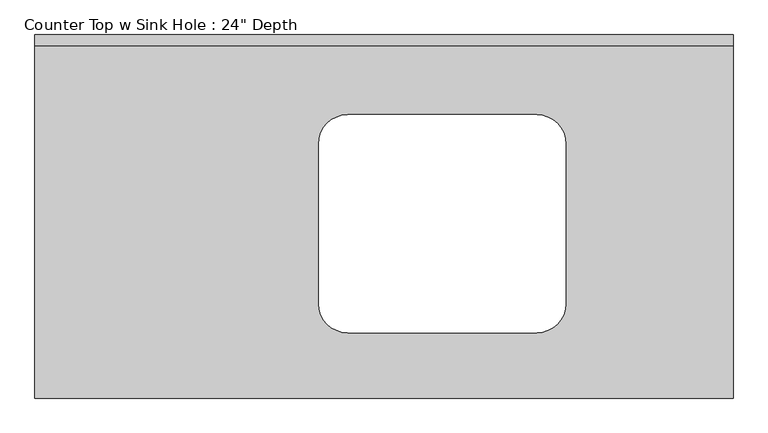
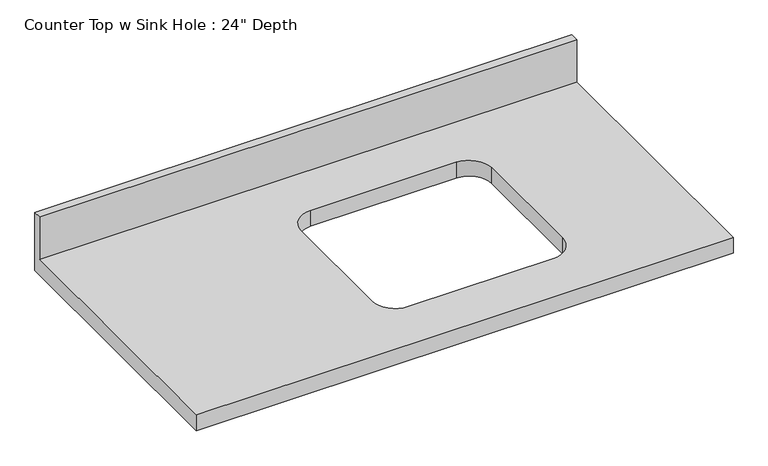
"""IFC4 building model written with IfcOpenShell, lengths in millimetres: furniture geometry."""

from ifc_helpers import new_model, si_unit, frame, origin, place, context, project, spatial, polyline, circle_curve, source, transform, mapped, element, save
from ifc_brep_helpers import plane_surface, revolved_surface, advanced_brep


def furniture_a1a13893(model_context):
    return source(origin(), model_context, "Body", "AdvancedBrep", [
        advanced_brep(
        [(-1200.4622951, -635.0, 914.4), (18.7377049, -635.0, 914.4), (18.7377049, -19.05, 914.4), (-1200.4622951, -19.05, 914.4), (-654.3622951, -139.7, 914.4), (-324.1622951, -139.7, 914.4), (-273.3622951, -190.5, 914.4), (-273.3622951, -469.9, 914.4), (-324.1622951, -520.7, 914.4), (-654.3622951, -520.7, 914.4), (-705.1622951, -469.9, 914.4), (-705.1622951, -190.5, 914.4), (18.7377049, 0.0, 876.3), (18.7377049, -635.0, 876.3), (-1200.4622951, -635.0, 876.3), (-1200.4622951, 0.0, 876.3), (-324.1622951, -139.7, 876.3), (-654.3622951, -139.7, 876.3), (-705.1622951, -190.5, 876.3), (-705.1622951, -469.9, 876.3), (-654.3622951, -520.7, 876.3), (-324.1622951, -520.7, 876.3), (-273.3622951, -469.9, 876.3), (-273.3622951, -190.5, 876.3), (-1200.4622951, 0.0, 1016.0), (18.7377049, 0.0, 1016.0), (-1200.4622951, -19.05, 1016.0), (18.7377049, -19.05, 1016.0)],
        [
            (0, 1),
            (1, 2),
            (2, 3),
            (3, 0),
            (4, 5),
            (5, 6, circle_curve(frame((-324.1622951, -190.5, 914.4), z_axis=(0.0, 0.0, -1.0), x_axis=(1.0, 0.0, 0.0)), 50.8)),
            (6, 7),
            (7, 8, circle_curve(frame((-324.1622951, -469.9, 914.4), z_axis=(0.0, 0.0, -1.0), x_axis=(1.0, 0.0, 0.0)), 50.8)),
            (8, 9),
            (9, 10, circle_curve(frame((-654.3622951, -469.9, 914.4), z_axis=(0.0, 0.0, -1.0), x_axis=(1.0, 0.0, 0.0)), 50.8)),
            (10, 11),
            (11, 4, circle_curve(frame((-654.3622951, -190.5, 914.4), z_axis=(0.0, 0.0, -1.0), x_axis=(1.0, 0.0, 0.0)), 50.8)),
            (12, 13),
            (13, 14),
            (14, 15),
            (15, 12),
            (16, 17),
            (17, 18, circle_curve(frame((-654.3622951, -190.5, 876.3), z_axis=(0.0, 0.0, 1.0), x_axis=(1.0, 0.0, 0.0)), 50.8)),
            (18, 19),
            (19, 20, circle_curve(frame((-654.3622951, -469.9, 876.3), z_axis=(0.0, 0.0, 1.0), x_axis=(1.0, 0.0, 0.0)), 50.8)),
            (20, 21),
            (21, 22, circle_curve(frame((-324.1622951, -469.9, 876.3), z_axis=(0.0, 0.0, 1.0), x_axis=(1.0, 0.0, 0.0)), 50.8)),
            (22, 23),
            (23, 16, circle_curve(frame((-324.1622951, -190.5, 876.3), z_axis=(0.0, 0.0, 1.0), x_axis=(1.0, 0.0, 0.0)), 50.8)),
            (15, 24),
            (24, 25),
            (25, 12),
            (14, 0),
            (3, 26),
            (26, 24),
            (13, 1),
            (25, 27),
            (27, 2),
            (4, 17),
            (16, 5),
            (11, 18),
            (10, 19),
            (9, 20),
            (8, 21),
            (7, 22),
            (6, 23),
            (26, 27),
        ],
        [
            plane_surface(frame((-1200.4622951, 0.0, 914.4), z_axis=(0.0, 0.0, 1.0), x_axis=(-1.0, 0.0, 0.0))),
            plane_surface(frame((-1200.4622951, 0.0, 876.3), z_axis=(0.0, 0.0, -1.0), x_axis=(1.0, 0.0, 0.0))),
            plane_surface(frame((18.7377049, 0.0, 914.4), z_axis=(0.0, 1.0, 0.0), x_axis=(0.0, 0.0, -1.0))),
            plane_surface(frame((-1200.4622951, 0.0, 914.4), z_axis=(-1.0, 0.0, 0.0), x_axis=(0.0, 0.0, -1.0))),
            plane_surface(frame((-1200.4622951, -635.0, 914.4), z_axis=(0.0, -1.0, 0.0), x_axis=(0.0, 0.0, -1.0))),
            plane_surface(frame((18.7377049, -635.0, 914.4), z_axis=(1.0, 0.0, 0.0), x_axis=(0.0, 0.0, -1.0))),
            plane_surface(frame((-324.1622951, -139.7, 914.4), z_axis=(0.0, -1.0, 0.0), x_axis=(0.0, 0.0, -1.0))),
            revolved_surface(polyline([(-603.5622951, -190.5, 914.4), (-603.5622951, -190.5, 876.3)]), (-654.3622951, -190.5, 876.3), (0.0, 0.0, 1.0)),
            plane_surface(frame((-705.1622951, -190.5, 914.4), z_axis=(1.0, 0.0, 0.0), x_axis=(0.0, 0.0, -1.0))),
            revolved_surface(polyline([(-603.5622951, -469.9, 914.4), (-603.5622951, -469.9, 876.3)]), (-654.3622951, -469.9, 876.3), (0.0, 0.0, 1.0)),
            plane_surface(frame((-654.3622951, -520.7, 914.4), z_axis=(0.0, 1.0, 0.0), x_axis=(0.0, 0.0, -1.0))),
            revolved_surface(polyline([(-273.3622951, -469.9, 914.4), (-273.3622951, -469.9, 876.3)]), (-324.1622951, -469.9, 876.3), (0.0, 0.0, 1.0)),
            plane_surface(frame((-273.3622951, -469.9, 914.4), z_axis=(-1.0, 0.0, 0.0), x_axis=(0.0, 0.0, -1.0))),
            revolved_surface(polyline([(-273.3622951, -190.5, 914.4), (-273.3622951, -190.5, 876.3)]), (-324.1622951, -190.5, 876.3), (0.0, 0.0, 1.0)),
            plane_surface(frame((-1200.4622951, 0.0, 1016.0), z_axis=(0.0, 0.0, 1.0), x_axis=(0.0, -1.0, 0.0))),
            plane_surface(frame((-1200.4622951, -19.05, 1016.0), z_axis=(0.0, -1.0, 0.0), x_axis=(0.0, 0.0, -1.0))),
        ],
        [
            (0, [[1, 2, 3, 4], [5, 6, 7, 8, 9, 10, 11, 12]]),
            (1, [[13, 14, 15, 16], [17, 18, 19, 20, 21, 22, 23, 24]]),
            (2, [[-16, 25, 26, 27]]),
            (3, [[-15, 28, -4, 29, 30, -25]]),
            (4, [[-1, -28, -14, 31]]),
            (5, [[-13, -27, 32, 33, -2, -31]]),
            (6, [[34, -17, 35, -5]]),
            (7, [[-34, -12, 36, -18]]),
            (8, [[-36, -11, 37, -19]]),
            (9, [[-37, -10, 38, -20]]),
            (10, [[-38, -9, 39, -21]]),
            (11, [[-39, -8, 40, -22]]),
            (12, [[-40, -7, 41, -23]]),
            (13, [[-35, -24, -41, -6]]),
            (14, [[-30, 42, -32, -26]]),
            (15, [[-42, -29, -3, -33]]),
        ],
    ),
    ])


if __name__ == "__main__":
    model = new_model("IFC4")
    model_context = context("Model", 3, world=origin())
    ifc_project = project(units=[si_unit("LENGTHUNIT", "METRE", prefix="MILLI")], contexts=[model_context])
    site = spatial("IfcSite", under=ifc_project)
    building = spatial("IfcBuilding", under=site)
    placement = place(None, origin())
    furniture_shape = furniture_a1a13893(model_context)
    element("IfcFurniture", 1, ObjectType="Counter Top w Sink Hole : 24\" Depth", at=placement, inside=building, context=model_context, shape_type="MappedRepresentation", body=[
        mapped(furniture_shape, transform((0.0, 0.0, 0.0), x_axis=(1.0, 0.0, 0.0), y_axis=(0.0, 1.0, 0.0), z_axis=(0.0, 0.0, 1.0))),
    ])
    save(model, "model.ifc")

# Revit data of these elements
# Type "Counter Top w Sink Hole : 24\" Depth"
#   Assembly Code = "C1030400"
#   Counter Thickness = 0' - 1 1/2"
#   Depth [instance default] = 2' - 1"
#   Height = 3' - 0"
#   Length [instance default] = 8' - 0"
#   Sink Location [instance default] = 2' - 0"
#   Sink Location To Wall [instance default] = 0' - 6"
#   Sink Opening Depth [instance default] = 1' - 3"
#   Sink Opening Width [instance default] = 2' - 3"
#   Counter Top Material = none
#   Default Elevation = 0
# Element 1 (IfcFurniture, "Counter Top w Sink Hole : 24\" Depth")
#   Length = 4' - 0"
#   Sink Location = 2' - 4"
#   Sink Opening Depth = 1' - 2"
#   Sink Opening Width = 1' - 4"
#   Materials on its faces: "Counter Top"
# Materials
#   "Counter Top": class "Wood", colour RGB 226 177 128, transparency 0
